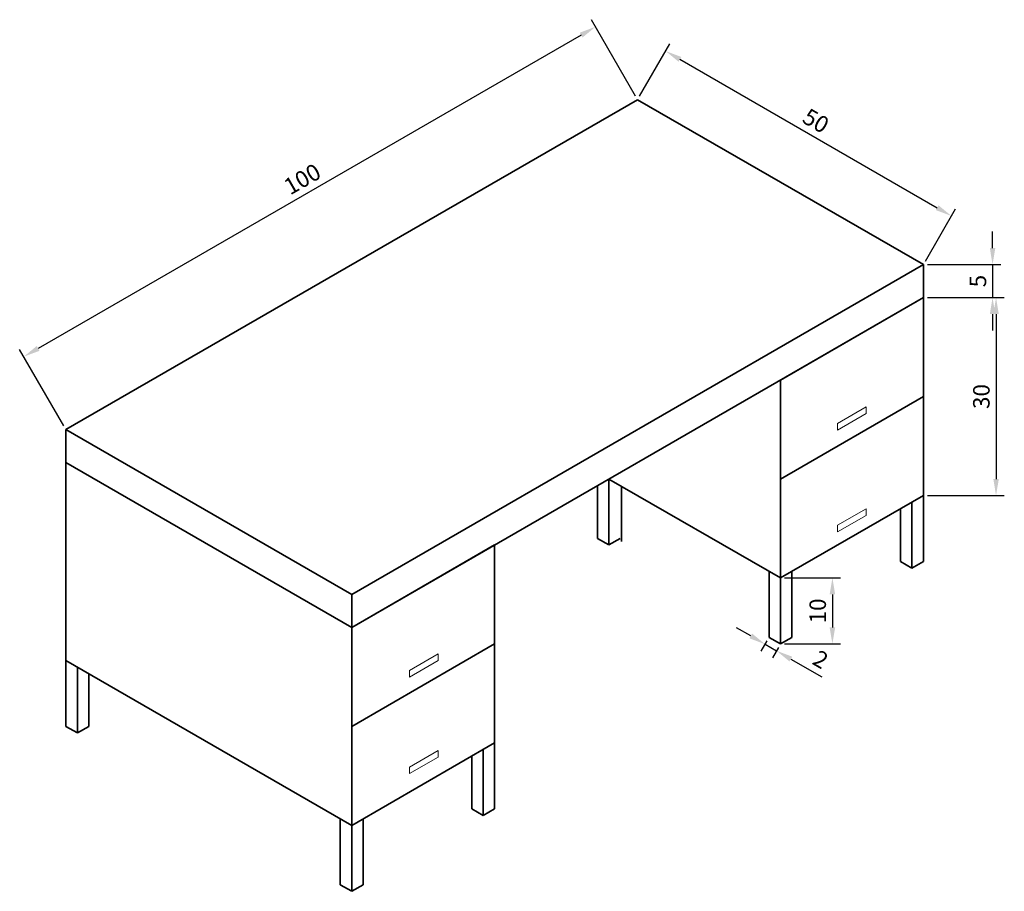
# Model space of a CAD drawing. Units: millimetres. Extents: x 2044 to 2193, y 1850 to 1983.
import ezdxf

# ---------------------------------------------------------------- set-up
doc = ezdxf.new("R2010")
doc.units = ezdxf.units.MM
for name, color, linetype, lineweight in [('A-ANNO-DIMS', 2, 'Continuous', 18), ('A-FURN', 7, 'Continuous', 35), ('A-FURN-HDWR', 8, 'Continuous', 18)]:
    doc.layers.add(name, color=color, linetype=linetype, lineweight=lineweight)
doc.styles.get("Standard").update_dxf_attribs({"font": 'arial.ttf'})
doc.dimstyles.new('ISO-25', dxfattribs={"dimtxt": 2.5, "dimasz": 2.5, "dimexe": 1.25, "dimexo": 0.625, "dimtad": 1, "dimtxsty": 'Standard', "dimcen": 2.5, "dimadec": 0, "dimazin": 0, "dimtfac": 1, "dimtmove": 0, "dimatfit": 3, "dimfxl": 1, "dimarcsym": 0})

# ---------------------------------------------------------------- blocks, each defined once
blk = doc.blocks.new('*D1')
at = {"layer": 'A-ANNO-DIMS', "color": 0, "lineweight": -2, "transparency": 16777216}
for p, q in [((2136.86, 1970.97), (2130.17, 1982.56)), ((2128.63, 1980.23), (2046.35, 1932.73)), ((2050.25, 1920.97), (2043.56, 1932.56))]:
    blk.add_line(p, q, dxfattribs=at)
at = {"layer": 'A-ANNO-DIMS', "color": 0, "transparency": 16777216}
for points in [[(2128.42, 1980.59), (2128.84, 1979.86), (2130.79, 1981.48)], [(2046.15, 1933.09), (2046.56, 1932.36), (2044.19, 1931.48)]]:
    blk.add_solid(points, dxfattribs=at)
at = {"layer": 'Defpoints', "color": 0, "transparency": 16777216}
for p in [(2137.17, 1970.43), (2044.19, 1931.48), (2050.57, 1920.43)]:
    blk.add_point(p, dxfattribs=at)
at = {"layer": 'A-ANNO-DIMS', "color": 0, "transparency": 16777216, "insert": (2086.54, 1958.12), "char_height": 2.5, "attachment_point": 5, "rotation": 30}
blk.add_mtext('100', dxfattribs=at)
blk = doc.blocks.new('*D2')
at = {"layer": 'A-ANNO-DIMS', "color": 0, "lineweight": -2, "transparency": 16777216}
for p, q in [((2137.48, 1970.97), (2142.05, 1978.88)), ((2143.59, 1976.55), (2182.56, 1954.05)), ((2180.78, 1945.97), (2185.35, 1953.88))]:
    blk.add_line(p, q, dxfattribs=at)
at = {"layer": 'A-ANNO-DIMS', "color": 0, "transparency": 16777216}
for points in [[(2143.8, 1976.91), (2143.38, 1976.19), (2141.43, 1977.8)], [(2182.77, 1954.41), (2182.36, 1953.69), (2184.73, 1952.8)]]:
    blk.add_solid(points, dxfattribs=at)
at = {"layer": 'Defpoints', "color": 0, "transparency": 16777216}
for p in [(2137.17, 1970.43), (2184.73, 1952.8), (2180.47, 1945.43)]:
    blk.add_point(p, dxfattribs=at)
at = {"layer": 'A-ANNO-DIMS', "color": 0, "transparency": 16777216, "insert": (2164.03, 1966.95), "char_height": 2.5, "attachment_point": 5, "rotation": 330}
blk.add_mtext('50', dxfattribs=at)
blk = doc.blocks.new('*D3')
at = {"layer": 'A-ANNO-DIMS', "color": 0, "lineweight": -2, "transparency": 16777216}
for p, q in [((2190.95, 1947.93), (2190.95, 1950.43)), ((2181.1, 1945.43), (2192.2, 1945.43)), ((2190.95, 1945.43), (2190.95, 1940.43)), ((2181.1, 1940.43), (2192.2, 1940.43)), ((2190.95, 1937.93), (2190.95, 1935.43))]:
    blk.add_line(p, q, dxfattribs=at)
at = {"layer": 'A-ANNO-DIMS', "color": 0, "transparency": 16777216}
for points in [[(2190.54, 1947.93), (2191.37, 1947.93), (2190.95, 1945.43)], [(2190.54, 1937.93), (2191.37, 1937.93), (2190.95, 1940.43)]]:
    blk.add_solid(points, dxfattribs=at)
at = {"layer": 'Defpoints', "color": 0, "transparency": 16777216}
for p in [(2180.47, 1945.43), (2180.47, 1940.43), (2190.95, 1940.43)]:
    blk.add_point(p, dxfattribs=at)
at = {"layer": 'A-ANNO-DIMS', "color": 0, "transparency": 16777216, "insert": (2189.06, 1942.93), "char_height": 2.5, "attachment_point": 5, "rotation": 90}
blk.add_mtext('5', dxfattribs=at)
blk = doc.blocks.new('*D4')
at = {"layer": 'A-ANNO-DIMS', "color": 0, "lineweight": -2, "transparency": 16777216}
for p, q in [((2181.1, 1940.43), (2192.73, 1940.43)), ((2191.48, 1937.93), (2191.48, 1912.93)), ((2181.1, 1910.43), (2192.73, 1910.43))]:
    blk.add_line(p, q, dxfattribs=at)
at = {"layer": 'A-ANNO-DIMS', "color": 0, "transparency": 16777216}
for points in [[(2191.07, 1937.93), (2191.9, 1937.93), (2191.48, 1940.43)], [(2191.07, 1912.93), (2191.9, 1912.93), (2191.48, 1910.43)]]:
    blk.add_solid(points, dxfattribs=at)
at = {"layer": 'Defpoints', "color": 0, "transparency": 16777216}
for p in [(2180.47, 1940.43), (2180.47, 1910.43), (2191.48, 1910.43)]:
    blk.add_point(p, dxfattribs=at)
at = {"layer": 'A-ANNO-DIMS', "color": 0, "transparency": 16777216, "insert": (2189.58, 1925.43), "char_height": 2.5, "attachment_point": 5, "rotation": 90}
blk.add_mtext('30', dxfattribs=at)
blk = doc.blocks.new('*D5')
at = {"layer": 'A-ANNO-DIMS', "color": 0, "lineweight": -2, "transparency": 16777216}
for p, q in [((2159.45, 1897.93), (2167.94, 1897.93)), ((2166.69, 1895.43), (2166.69, 1890.43)), ((2159.45, 1887.93), (2167.94, 1887.93))]:
    blk.add_line(p, q, dxfattribs=at)
at = {"layer": 'A-ANNO-DIMS', "color": 0, "transparency": 16777216}
for points in [[(2166.27, 1895.43), (2167.11, 1895.43), (2166.69, 1897.93)], [(2166.27, 1890.43), (2167.11, 1890.43), (2166.69, 1887.93)]]:
    blk.add_solid(points, dxfattribs=at)
at = {"layer": 'Defpoints', "color": 0, "transparency": 16777216}
for p in [(2158.82, 1897.93), (2158.82, 1887.93), (2166.69, 1887.93)]:
    blk.add_point(p, dxfattribs=at)
at = {"layer": 'A-ANNO-DIMS', "color": 0, "transparency": 16777216, "insert": (2164.79, 1892.93), "char_height": 2.5, "attachment_point": 5, "rotation": 90}
blk.add_mtext('10', dxfattribs=at)
blk = doc.blocks.new('*D6')
at = {"layer": 'A-ANNO-DIMS', "color": 0, "lineweight": -2, "transparency": 16777216}
for p, q in [((2154.33, 1889.14), (2152.16, 1890.39)), ((2156.78, 1888.39), (2155.87, 1886.81)), ((2156.49, 1887.89), (2158.22, 1886.89)), ((2158.51, 1887.39), (2157.6, 1885.81)), ((2160.39, 1885.64), (2165.07, 1882.94))]:
    blk.add_line(p, q, dxfattribs=at)
at = {"layer": 'A-ANNO-DIMS', "color": 0, "transparency": 16777216}
for points in [[(2154.53, 1889.5), (2154.12, 1888.78), (2156.49, 1887.89)], [(2160.6, 1886), (2160.18, 1885.28), (2158.22, 1886.89)]]:
    blk.add_solid(points, dxfattribs=at)
at = {"layer": 'Defpoints', "color": 0, "transparency": 16777216}
for p in [(2157.09, 1888.93), (2158.82, 1887.93), (2158.22, 1886.89)]:
    blk.add_point(p, dxfattribs=at)
at = {"layer": 'A-ANNO-DIMS', "color": 0, "transparency": 16777216, "insert": (2164.75, 1885.3), "char_height": 2.5, "attachment_point": 5, "rotation": 330}
blk.add_mtext('2', dxfattribs=at)
blk = doc.blocks.new('DRAWER-PULL')
for p, q in [((4.33, 3.5), (0, 1)), ((4.33, 2.5), (4.33, 3.5)), ((0, 0), (4.33, 2.5)), ((0, 1), (0, 0))]:
    blk.add_line(p, q)

msp = doc.modelspace()

# ---------------------------------------------------------------- linework, layer by layer
at = {"layer": 'A-FURN'}
for p, q in [((2050.567, 1920.428), (2137.17, 1970.428)), ((2137.17, 1970.428), (2180.471, 1945.428)), ((2180.471, 1945.428), (2093.869, 1895.428)), ((2180.471, 1940.428), (2180.471, 1945.428)), ((2180.471, 1945.428), (2180.471, 1940.428)), ((2093.869, 1890.428), (2180.471, 1940.428)), ((2180.471, 1940.428), (2158.82, 1927.928)), ((2180.471, 1940.428), (2180.471, 1910.428)), ((2180.471, 1940.428), (2180.471, 1925.428)), ((2158.82, 1927.928), (2158.82, 1897.928)), ((2180.471, 1925.428), (2158.82, 1912.928)), ((2093.869, 1895.428), (2050.567, 1920.428)), ((2050.567, 1920.428), (2050.567, 1915.428)), ((2050.567, 1915.428), (2050.567, 1885.428)), ((2093.869, 1890.428), (2050.567, 1915.428)), ((2158.82, 1897.928), (2132.84, 1912.928)), ((2132.84, 1912.928), (2132.84, 1902.928)), ((2131.108, 1903.928), (2131.108, 1911.928)), ((2134.762, 1903.48), (2134.762, 1911.818)), ((2180.471, 1910.428), (2158.82, 1897.928)), ((2178.739, 1899.428), (2178.739, 1909.428)), ((2180.471, 1910.428), (2180.471, 1900.428)), ((2180.471, 1900.428), (2180.471, 1910.428)), ((2177.007, 1900.428), (2177.007, 1908.428)), ((2132.84, 1902.928), (2131.108, 1903.928)), ((2132.822, 1902.928), (2134.554, 1903.928)), ((2093.869, 1890.428), (2115.519, 1902.928)), ((2115.519, 1902.928), (2115.519, 1872.928)), ((2178.739, 1899.428), (2177.007, 1900.428)), ((2180.471, 1900.428), (2178.739, 1899.428)), ((2157.088, 1888.928), (2157.088, 1898.928)), ((2160.553, 1888.928), (2160.553, 1898.928)), ((2158.82, 1897.928), (2158.82, 1887.928)), ((2093.869, 1895.428), (2093.869, 1890.428)), ((2093.869, 1860.428), (2093.869, 1890.428)), ((2158.82, 1887.928), (2157.088, 1888.928)), ((2158.82, 1887.928), (2160.553, 1888.928)), ((2115.519, 1887.928), (2093.869, 1875.428)), ((2050.567, 1885.428), (2050.567, 1875.428)), ((2050.567, 1885.428), (2093.869, 1860.428)), ((2052.299, 1874.428), (2052.299, 1884.428)), ((2054.031, 1875.428), (2054.031, 1883.428)), ((2050.567, 1875.428), (2052.299, 1874.428)), ((2052.299, 1874.428), (2054.031, 1875.428)), ((2115.519, 1872.928), (2093.869, 1860.428)), ((2115.519, 1872.928), (2115.519, 1862.928)), ((2112.055, 1862.928), (2112.055, 1870.928)), ((2113.787, 1861.928), (2113.787, 1871.928)), ((2113.787, 1861.928), (2112.055, 1862.928)), ((2115.519, 1862.928), (2113.787, 1861.928)), ((2092.137, 1851.428), (2092.137, 1861.428)), ((2093.869, 1860.428), (2093.869, 1850.428)), ((2095.601, 1851.428), (2095.601, 1861.428)), ((2093.869, 1850.428), (2092.137, 1851.428)), ((2093.869, 1850.428), (2095.601, 1851.428))]:
    msp.add_line(p, q, dxfattribs=at)

# ---------------------------------------------------------------- block references
at = {"layer": 'A-FURN-HDWR'}
for p in [(2167.481, 1920.35), (2167.481, 1904.92), (2102.64, 1882.914), (2102.64, 1868.267)]:
    msp.add_blockref('DRAWER-PULL', p, dxfattribs=at)

# ---------------------------------------------------------------- dimensions: what is measured, and where the dimension line sits
at = {"layer": 'A-ANNO-DIMS'}
for p1, p2, distance, picture, middle in [((2137.17, 1970.428), (2050.567, 1920.428), -12.756, '*D1', (2086.54, 1958.122)), ((2137.17, 1970.428), (2180.471, 1945.428), 8.515, '*D2', (2164.029, 1966.949)), ((2180.471, 1945.428), (2180.471, 1940.428), 10.482, '*D3', (2189.057, 1942.928)), ((2180.471, 1940.428), (2180.471, 1910.428), 11.011, '*D4', (2189.58, 1925.428)), ((2158.82, 1897.928), (2158.82, 1887.928), 7.868, '*D5', (2164.787, 1892.928)), ((2157.088, 1888.928), (2158.82, 1887.928), -1.194, '*D6', (2164.752, 1885.296))]:
    dim = msp.add_aligned_dim(p1=p1, p2=p2, distance=distance, dimstyle='ISO-25', override={"dimclrd": 0, "dimclre": 0, "dimclrt": 0}, dxfattribs=at)
    dim.commit()
    dim.dimension.update_dxf_attribs({"geometry": picture, "text_midpoint": middle})

doc.saveas('drawing.dxf')
